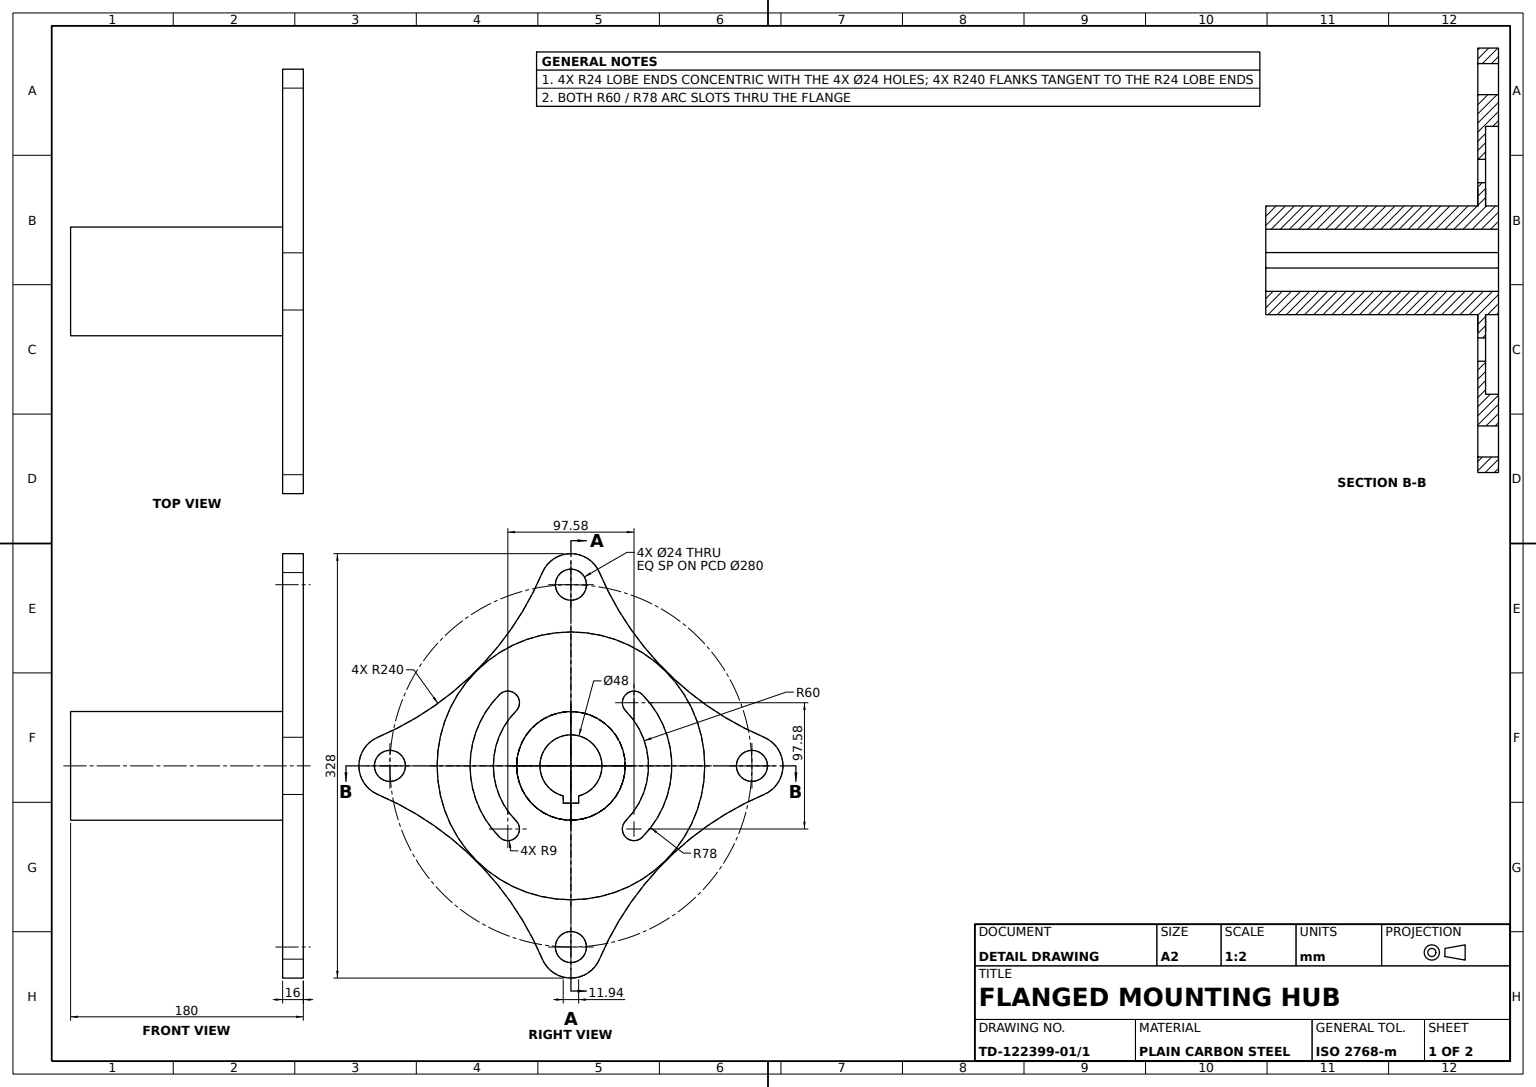
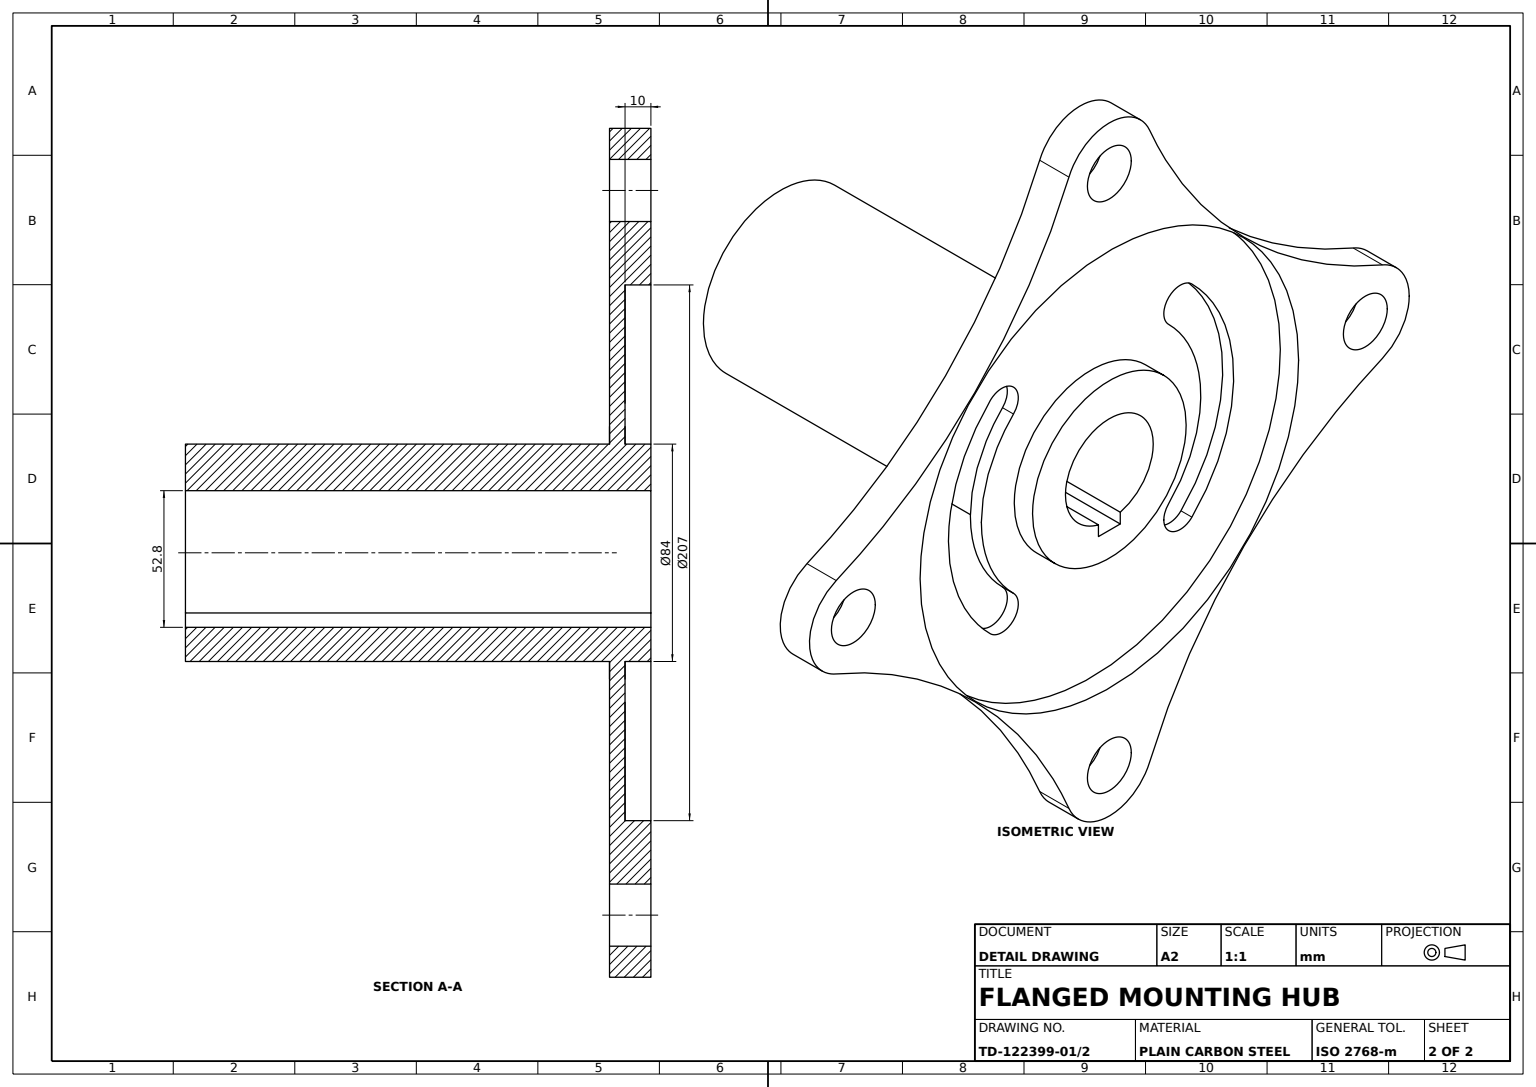
SolidWorks part; units mm, degrees
material "Plain Carbon Steel"
ref_plane "Front Plane" through (0, 0, 0) normal (0, 0, 1) x (1, 0, 0)
ref_plane "Top Plane" through (0, 0, 0) normal (0, 1, 0) x (1, 0, 0)
ref_plane "Right Plane" through (0, 0, 0) normal (1, 0, 0) x (0, 0, -1)
sketch "Square Flange Profile Sketch" plane through (0, 0, 0) normal (0, 1, 0) x (1, 0, 0)
  line L0 (0, 0) -> (0, 100.5) construction
  line L1 (0, 0) -> (-236.3464, 0) construction
  circle A6 centre (0, 140) radius 12
  arc A7 (22.0959, 149.3686) -> (-22.0959, 149.3686) centre (0, 140) ccw
  circle A8 centre (140, 0) radius 12
  arc A9 (149.3686, -22.0959) -> (149.3686, 22.0959) centre (140, 0) ccw
  circle A10 centre (0, -140) radius 12
  arc A11 (-22.0959, -149.3686) -> (22.0959, -149.3686) centre (0, -140) ccw
  circle A12 centre (-140, 0) radius 12
  arc A13 (-149.3686, 22.0959) -> (-149.3686, -22.0959) centre (-140, 0) ccw
  arc A14 (-149.3686, 22.0959) -> (-22.0959, 149.3686) centre (-243.0549, 243.0549) ccw
  arc A15 (149.3686, 22.0959) -> (22.0959, 149.3686) centre (243.0549, 243.0549) cw
  arc A16 (149.3686, -22.0959) -> (22.0959, -149.3686) centre (243.0549, -243.0549) ccw
  arc A17 (-149.3686, -22.0959) -> (-22.0959, -149.3686) centre (-243.0549, -243.0549) cw
  point P19 (0, 0)
  dimension "D2" = 240
  dimension "D3" = 24
  dimension "D4" = 48
  dimension "D7" = 140
  dimension "D5" = 4
extrude "Square Flange 240x16" add sketch "Square Flange Profile Sketch" along normal blind 16
sketch "Flange Step Circle Sketch" plane through (0, 16, 0) normal (0, 1, 0) x (1, 0, 0)
  circle A0 centre (0, 0) radius 103.5
  dimension "D1" = 207
  dimension "D2" = 149.3686
  dimension "D3" = 149.3686
extrude "Flange Step Cut Ø207" cut sketch "Flange Step Circle Sketch" against normal blind 10
sketch "Arc Slots Sketch" plane through (0, 6, 0) normal (0, 1, 0) x (1, 0, 0)
  line L0 (0, 0) -> (-120.5955, 120.5955) construction
  line L1 (0, 0) -> (0, 179.3919) construction
  line L2 (0, 0) -> (139.8934, 139.8934) construction
  line L3 (0, 0) -> (220.6246, 0) construction
  arc A0 (55.1543, 55.1543) -> (-55.1543, 55.1543) centre (0, 0) ccw
  arc A1 (42.4264, 42.4264) -> (-42.4264, 42.4264) centre (0, 0) ccw
  arc A2 (42.4264, 42.4264) -> (55.1543, 55.1543) centre (48.7904, 48.7904) ccw
  arc A3 (-55.1543, 55.1543) -> (-42.4264, 42.4264) centre (-48.7904, 48.7904) ccw
  arc A4 (42.4264, -42.4264) -> (-42.4264, -42.4264) centre (0, 0) cw
  arc A5 (-55.1543, -55.1543) -> (-42.4264, -42.4264) centre (-48.7904, -48.7904) cw
  arc A6 (55.1543, -55.1543) -> (-55.1543, -55.1543) centre (0, 0) cw
  arc A7 (42.4264, -42.4264) -> (55.1543, -55.1543) centre (48.7904, -48.7904) cw
  dimension "D1" = 45
  dimension "D3" = 18
  dimension "D4" = 78
  dimension "D2" = 45
extrude "Arc Slots R78" cut sketch "Arc Slots Sketch" against normal blind 60
sketch "Hub Sketch" plane through (0, 16, 0) normal (0, 1, 0) x (1, 0, 0)
  circle A0 centre (0, 0) radius 42
  dimension "D1" = 84
extrude "Hub Ø84" add sketch "Hub Sketch" against normal blind 180 contours A0
sketch "Bore Sketch" plane through (0, 16, 0) normal (0, 1, 0) x (1, 0, 0)
  circle A0 centre (0, 0) radius 24
  dimension "D1" = 48
extrude "Bore Ø48" cut sketch "Bore Sketch" against normal blind 180 contours A0
sketch "Keyway Sketch" plane through (0, 16, 0) normal (0, 1, 0) x (1, 0, 0)
  line L1 (23.2456, 5.97) -> (28.7956, 5.97)
  line L2 (23.2456, 5.97) -> (23.2456, -5.97)
  line L3 (23.2456, -5.97) -> (28.7956, -5.97)
  line L4 (28.7956, 5.97) -> (28.7956, -5.97)
  circle A0 centre (0, 0) radius 24 construction
  point P7 (23.2456, 0)
  dimension "D1" = 11.94
  dimension "D2" = 5.55
extrude "Keyway" cut sketch "Keyway Sketch" against normal blind 180
